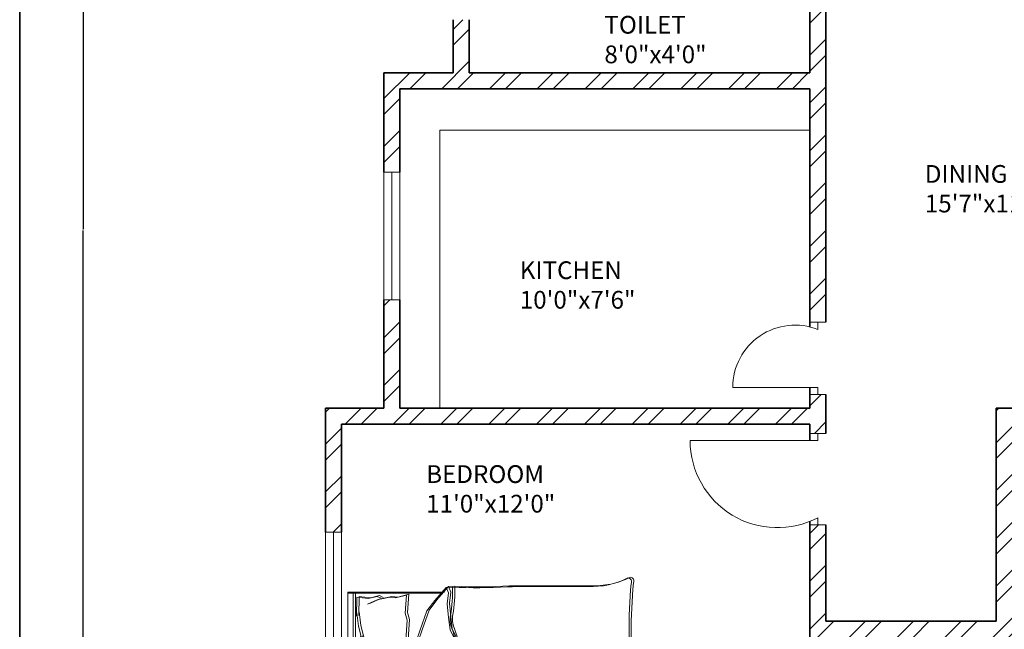
# Model space of a CAD drawing. Units: inches. Extents: x 1885 to 2748, y 783 to 2421.
# Tile 20 of 117: x 1885 to 2163, y 1178 to 1350. Entities that reach past the tile are written whole.
import ezdxf

# ---------------------------------------------------------------- set-up
doc = ezdxf.new("R2010")
doc.units = ezdxf.units.IN
for name, color, linetype, lineweight in [('A-ANNO-DIMS', 2, 'Continuous', 18), ('A-ANNO-TTLB', 7, 'Continuous', 35), ('A-AREA-IDEN', 7, 'Continuous', 18), ('A-DOOR', 31, 'Continuous', 18), ('A-FLOR-CASE', 9, 'Continuous', 18), ('A-FURN', 8, 'Continuous', 13), ('A-GLAZ', 181, 'Continuous', 18), ('A-WALL', 7, 'Continuous', 35)]:
    doc.layers.add(name, color=color, linetype=linetype, lineweight=lineweight)
doc.layers.add('A-WALL-PATT', color=85, linetype='Continuous', lineweight=13, true_color=0x58ba48)
doc.styles.get("Standard").update_dxf_attribs({"font": 'arial.ttf'})
doc.dimstyles.get("Standard").update_dxf_attribs({"dimtxt": 0.18, "dimasz": 0.18, "dimexe": 0.18, "dimexo": 0.0625, "dimgap": 0.09, "dimtad": 0, "dimtih": 1, "dimtoh": 1, "dimdec": 4, "dimzin": 0, "dimdsep": 46, "dimtxsty": 'Standard', "dimcen": 0.09, "dimadec": 0, "dimazin": 0, "dimtfac": 1, "dimtdec": 4, "dimtofl": 0, "dimtmove": 0, "dimatfit": 3, "dimfxl": 1, "dimtolj": 1, "dimtzin": 0, "dimarcsym": 0})

# ---------------------------------------------------------------- blocks, each defined once
blk = doc.blocks.new('BED-DOUBLE')
for p, q in [((27.75, 52.87), (24.5, 49.16)), ((27.75, 52.87), (24.5, 49.16)), ((28.39, 53.09), (25.14, 49.39)), ((28.39, 53.09), (25.14, 49.39)), ((29.49, 52.95), (27.75, 52.87, 3.87)), ((29.49, 52.95), (27.75, 52.87, 3.87)), ((28.37, 51.33), (27.75, 52.87)), ((28.37, 51.33), (27.75, 52.87)), ((30.13, 53.17), (28.39, 53.09, 3.87)), ((30.13, 53.17), (28.39, 53.09, 3.87)), ((29.01, 51.56), (28.39, 53.09)), ((29.01, 51.56), (28.39, 53.09)), ((0, 51.49), (0.64, 51.49)), ((0, 3.47), (0, 51.49)), ((0, 51.26), (26.61, 51.26)), ((0, 51.26), (26.61, 51.26)), ((0.64, 51.49), (27.25, 51.49)), ((0.64, 51.49), (27.25, 51.49)), ((1.54, 3.47), (1.54, 51.26)), ((1.54, 3.47), (1.54, 51.26)), ((2.18, 3.7), (2.18, 51.49)), ((2.18, 3.7), (2.18, 51.49)), ((2.56, 50.11), (2.46, 44.71)), ((2.56, 50.11), (2.46, 44.71)), ((2.56, 50.11), (5.77, 49.73)), ((2.56, 50.11), (5.77, 49.73)), ((3.2, 50.34), (3.1, 44.94)), ((3.2, 50.34), (3.1, 44.94)), ((3.2, 50.34), (6.41, 49.96)), ((3.2, 50.34), (6.41, 49.96)), ((5.77, 49.73), (8.34, 50.33)), ((5.77, 49.73), (8.34, 50.33)), ((6.41, 49.96), (8.98, 50.56)), ((6.41, 49.96), (8.98, 50.56)), ((11.83, 50.11), (8.26, 49.31)), ((11.83, 50.11), (8.26, 49.31)), ((8.34, 50.33), (9.39, 49.81)), ((8.34, 50.33), (9.39, 49.81)), ((12.47, 50.34), (8.9, 49.54)), ((12.47, 50.34), (8.9, 49.54)), ((8.98, 50.56), (10.03, 50.04)), ((8.98, 50.56), (10.03, 50.04)), ((13.44, 49.92), (11.83, 50.11)), ((13.44, 49.92), (11.83, 50.11)), ((14.08, 50.15), (12.47, 50.34)), ((14.08, 50.15), (12.47, 50.34)), ((16.58, 50.7), (13.44, 49.92)), ((16.58, 50.7), (13.44, 49.92)), ((17.22, 50.93), (14.08, 50.15)), ((17.22, 50.93), (14.08, 50.15)), ((16.17, 45.57), (16.58, 50.7)), ((16.17, 45.56), (16.58, 50.7)), ((16.81, 45.79), (17.22, 50.93)), ((16.81, 45.79), (17.22, 50.93)), ((28.06, 48.23), (28.37, 51.33)), ((28.06, 48.23), (28.37, 51.33)), ((28.7, 48.46), (29.01, 51.56)), ((28.7, 48.46), (29.01, 51.56)), ((8.26, 49.31), (5.58, 48.13)), ((8.26, 49.31), (5.58, 48.13)), ((8.9, 49.54), (6.22, 48.36)), ((8.9, 49.54), (6.22, 48.36)), ((24.5, 49.16), (22.33, 46.22)), ((24.5, 49.16), (22.33, 46.22)), ((25.14, 49.39), (22.97, 46.45)), ((25.14, 49.39), (22.97, 46.45)), ((28.37, 44.36), (28.06, 48.23)), ((28.37, 44.36), (28.06, 48.23)), ((29.01, 44.59), (28.7, 48.46)), ((29.01, 44.59), (28.7, 48.46)), ((2.46, 44.71), (2.55, 45.71)), ((2.46, 44.71), (2.55, 45.71)), ((2.55, 45.71), (3.07, 41.91)), ((2.55, 45.71), (3.07, 41.91)), ((3.1, 44.94), (3.19, 45.94)), ((3.1, 44.94), (3.19, 45.94)), ((3.19, 45.94), (3.71, 42.14)), ((3.19, 45.94), (3.71, 42.14)), ((16.73, 43.6), (16.17, 45.57)), ((16.73, 43.6), (16.17, 45.56)), ((17.37, 43.83), (16.81, 45.79)), ((17.37, 43.83), (16.81, 45.79)), ((22.33, 46.22), (20.32, 40.64)), ((22.33, 46.22), (20.32, 40.64)), ((22.97, 46.45), (20.96, 40.87)), ((22.97, 46.45), (20.96, 40.87)), ((29.47, 41.18), (29.01, 44.59)), ((29.47, 41.18), (29.01, 44.59)), ((3.07, 41.91), (4.43, 36.49)), ((3.07, 41.91), (4.43, 36.49)), ((3.71, 42.14), (5.07, 36.72)), ((3.71, 42.14), (5.07, 36.72)), ((16.3, 36.59), (16.73, 43.6)), ((16.3, 36.59), (16.73, 43.6)), ((16.94, 36.82), (17.37, 43.83)), ((16.94, 36.82), (17.37, 43.83)), ((28.83, 40.95), (28.37, 44.36)), ((28.83, 40.95), (28.37, 44.36)), ((3.68, 39.2), (3.08, 37.13)), ((3.68, 39.2), (3.08, 37.13)), ((4.32, 39.43), (3.72, 37.36)), ((4.32, 39.43), (3.72, 37.36)), ((20.32, 40.64), (17.39, 32.3)), ((20.32, 40.64), (17.39, 32.3)), ((20.96, 40.87), (18.03, 32.53)), ((20.96, 40.87), (18.03, 32.53)), ((29.76, 38.94), (28.83, 40.95)), ((29.76, 38.94), (28.83, 40.95)), ((30.4, 39.17), (29.47, 41.18)), ((30.4, 39.17), (29.47, 41.18)), ((30.38, 36.46), (29.76, 38.94)), ((30.38, 36.46), (29.76, 38.94)), ((31.02, 36.69), (30.4, 39.17)), ((31.02, 36.69), (30.4, 39.17)), ((79.25, 15.06), (79.25, 39.68)), ((79.25, 15.06), (79.25, 39.68)), ((79.89, 15.29), (79.89, 39.9)), ((79.89, 15.29), (79.89, 39.9)), ((3.08, 37.13), (2.54, 34.2)), ((3.08, 37.13), (2.54, 34.2)), ((3.72, 37.36), (3.18, 34.43)), ((3.72, 37.36), (3.18, 34.43)), ((15.63, 32.56), (16.3, 36.59)), ((15.63, 32.56), (16.3, 36.59)), ((16.27, 32.79), (16.94, 36.82)), ((16.27, 32.79), (16.94, 36.82)), ((23.88, 34.45), (28.37, 36.15)), ((23.88, 34.45), (28.37, 36.15)), ((24.52, 34.68), (29.01, 36.38)), ((24.52, 34.68), (29.01, 36.38)), ((28.37, 36.15), (30.38, 36.46)), ((28.37, 36.15), (30.38, 36.46)), ((29.01, 36.38), (31.02, 36.69)), ((29.01, 36.38), (31.02, 36.69)), ((2.54, 34.2), (2.56, 33.88)), ((2.54, 34.2), (2.56, 33.88)), ((2.56, 33.88), (2.98, 29.45)), ((2.56, 33.88), (2.98, 29.45)), ((3.18, 34.43), (3.2, 34.11)), ((3.18, 34.43), (3.2, 34.11)), ((3.2, 34.11), (3.62, 29.68)), ((3.2, 34.11), (3.62, 29.68)), ((16.74, 30.75), (15.46, 33.82)), ((16.74, 30.75), (15.46, 33.82)), ((17.38, 30.98), (16.1, 34.05)), ((17.38, 30.98), (16.1, 34.05)), ((17.39, 30.26), (23.88, 34.45)), ((17.39, 30.26), (23.88, 34.45)), ((18.03, 30.49), (24.52, 34.68)), ((18.03, 30.49), (24.52, 34.68)), ((16.9, 28.3), (16.74, 30.75)), ((16.9, 28.3), (16.74, 30.75)), ((17.54, 28.52), (17.38, 30.98)), ((17.54, 28.52), (17.38, 30.98)), ((2.98, 29.45), (2.5, 27.98)), ((2.98, 29.45), (2.5, 27.98)), ((2.5, 27.98), (7.87, 27.73)), ((2.5, 27.98), (7.87, 27.73)), ((3.62, 29.68), (3.13, 28.2)), ((3.62, 29.68), (3.13, 28.2)), ((3.13, 28.2), (8.51, 27.96)), ((3.13, 28.2), (8.51, 27.96)), ((8.51, 27.96), (11.72, 27.58)), ((8.51, 27.96), (11.72, 27.58)), ((12.38, 27.43), (14.22, 28.13)), ((12.38, 27.43), (14.22, 28.13)), ((13.02, 27.66), (14.86, 28.36)), ((13.02, 27.66), (14.86, 28.36)), ((14.22, 28.13), (16.9, 28.3)), ((14.22, 28.13), (16.9, 28.3)), ((14.86, 28.36), (17.54, 28.52)), ((14.86, 28.36), (17.54, 28.52)), ((1.87, 25.98), (7.22, 26.56)), ((1.87, 25.98), (7.22, 26.56)), ((2.45, 24.54), (1.87, 25.98)), ((2.45, 24.54), (1.87, 25.98)), ((2.51, 26.21), (7.86, 26.79)), ((2.51, 26.21), (7.86, 26.79)), ((3.09, 24.76), (2.51, 26.21)), ((3.09, 24.76), (2.51, 26.21)), ((7.22, 26.56), (10.4, 27.14)), ((7.22, 26.56), (10.4, 27.14)), ((7.86, 26.79), (11.04, 27.37)), ((7.86, 26.79), (11.04, 27.37)), ((7.87, 27.73), (11.08, 27.35)), ((7.87, 27.73), (11.08, 27.35)), ((10.4, 27.14), (11.71, 27.14)), ((10.4, 27.14), (11.71, 27.14)), ((11.04, 27.37), (12.35, 27.37)), ((11.04, 27.37), (12.35, 27.37)), ((11.08, 27.35), (12.38, 27.43)), ((11.08, 27.35), (12.38, 27.43)), ((11.71, 27.14), (13.59, 26.56)), ((11.71, 27.14), (13.59, 26.56)), ((11.72, 27.58), (13.02, 27.66)), ((11.72, 27.58), (13.02, 27.66)), ((12.35, 27.37), (14.22, 26.79)), ((12.35, 27.37), (14.22, 26.79)), ((13.59, 26.56), (16.27, 26.56)), ((13.59, 26.56), (16.27, 26.56)), ((14.22, 26.79), (16.91, 26.79)), ((14.22, 26.79), (16.91, 26.79)), ((16.27, 26.56), (16.27, 24.1)), ((16.27, 26.56), (16.27, 24.1)), ((16.91, 26.79), (16.91, 24.33)), ((16.91, 26.79), (16.91, 24.33)), ((2.31, 20.09), (2.45, 24.54)), ((2.31, 20.09), (2.45, 24.54)), ((2.95, 20.32), (3.09, 24.76)), ((2.95, 20.32), (3.09, 24.76)), ((16.27, 24.1), (15.18, 20.96)), ((16.27, 24.1), (15.18, 20.96)), ((16.91, 24.33), (15.82, 21.19)), ((16.91, 24.33), (15.82, 21.19)), ((16.17, 19.38), (16.58, 24.51)), ((16.17, 19.38), (16.58, 24.51)), ((16.81, 19.61), (17.22, 24.74)), ((16.81, 19.61), (17.22, 24.74)), ((2.31, 19.77), (2.31, 20.09)), ((2.31, 19.77), (2.31, 20.09)), ((3.03, 16.88), (2.31, 19.77)), ((3.03, 16.88), (2.31, 19.77)), ((2.95, 20), (2.95, 20.32)), ((2.95, 20), (2.95, 20.32)), ((3.67, 17.11), (2.95, 20)), ((3.67, 17.11), (2.95, 20)), ((17.37, 17.65), (16.81, 19.61)), ((17.37, 17.65), (16.81, 19.61)), ((3.75, 14.85), (3.03, 16.88)), ((3.75, 14.85), (3.03, 16.88)), ((3.32, 12.11), (4.33, 17.6)), ((3.32, 12.11), (4.33, 17.6)), ((4.39, 15.08), (3.67, 17.11)), ((4.39, 15.08), (3.67, 17.11)), ((3.96, 12.34), (4.97, 17.83)), ((3.96, 12.34), (4.97, 17.83)), ((16.73, 17.42), (16.17, 19.38)), ((16.73, 17.42), (16.17, 19.38)), ((16.3, 10.41), (16.73, 17.42)), ((16.3, 10.41), (16.73, 17.42)), ((16.94, 10.64), (17.37, 17.65)), ((16.94, 10.64), (17.37, 17.65)), ((3.03, 8.28), (3.32, 12.11)), ((3.03, 8.28), (3.32, 12.11)), ((3.67, 8.51), (3.96, 12.34)), ((3.67, 8.51), (3.96, 12.34)), ((3.65, 8.41), (3.67, 8.51)), ((3.65, 8.41), (3.67, 8.51)), ((3.98, 4.13), (3.65, 8.41)), ((3.98, 4.13), (3.65, 8.41)), ((15.63, 6.38), (16.3, 10.41)), ((15.63, 6.38), (16.3, 10.41)), ((16.27, 6.61), (16.94, 10.64)), ((16.27, 6.61), (16.94, 10.64)), ((16.3, 10.41), (16.62, 9.28)), ((16.3, 10.41), (16.62, 9.28)), ((16.62, 9.28), (17.34, 4.18)), ((16.62, 9.28), (17.34, 4.18)), ((16.94, 10.64), (17.26, 9.51)), ((16.94, 10.64), (17.26, 9.51)), ((17.26, 9.51), (17.98, 4.41)), ((17.26, 9.51), (17.98, 4.41)), ((3.01, 8.18), (3.03, 8.28)), ((3.01, 8.18), (3.03, 8.28)), ((3.34, 3.9), (3.01, 8.18)), ((3.34, 3.9), (3.01, 8.18)), ((8.96, 5.05), (6.21, 6.06)), ((8.96, 5.05), (6.21, 6.06)), ((9.6, 5.28), (6.85, 6.29)), ((9.6, 5.28), (6.85, 6.29)), ((18.11, 3.47), (0, 3.47)), ((18.11, 3.47), (0, 3.47)), ((18.75, 3.7), (0.64, 3.7)), ((18.75, 3.7), (0.64, 3.7)), ((3.32, 3.89), (6.5, 4.47)), ((3.32, 3.89), (6.5, 4.47)), ((3.96, 4.12), (7.14, 4.7)), ((3.96, 4.12), (7.14, 4.7)), ((6.5, 4.47), (9.1, 4.04)), ((6.5, 4.47), (9.1, 4.04)), ((7.14, 4.7), (9.74, 4.27)), ((7.14, 4.7), (9.74, 4.27)), ((12.57, 4.47), (8.96, 5.05)), ((12.57, 4.47), (8.96, 5.05)), ((9.1, 4.04), (10.12, 4.62)), ((9.1, 4.04), (10.12, 4.62)), ((13.21, 4.7), (9.6, 5.28)), ((13.21, 4.7), (9.6, 5.28)), ((9.74, 4.27), (10.75, 4.84)), ((9.74, 4.27), (10.75, 4.84)), ((14.16, 4.76), (12.57, 4.47)), ((14.16, 4.76), (12.57, 4.47)), ((14.8, 4.99), (13.21, 4.7)), ((14.8, 4.99), (13.21, 4.7)), ((17.34, 4.18), (14.16, 4.76)), ((17.34, 4.18), (14.16, 4.76)), ((17.98, 4.41), (14.8, 4.99)), ((17.98, 4.41), (14.8, 4.99))]:
    blk.add_line(p, q)
for centre, radius, start, end in [((68.67, 76.16), 23.07, 267.4714, 296.4681), ((68.67, 76.16), 23.07, 267.4714, 296.4681), ((69.31, 76.38), 23.07, 267.4714, 296.4681), ((69.31, 76.38), 23.07, 267.4714, 296.4681), ((78.87, 54.41), 1.1, 332.6588, 86.02), ((78.87, 54.41), 1.1, 332.6588, 86.02), ((79.51, 54.64), 1.1, 332.6588, 86.02), ((79.51, 54.64), 1.1, 332.6588, 86.02), ((-6.65, 51.33), 36.18, 349.8763, 2.5657), ((-6.65, 51.33), 36.18, 349.8763, 2.5657), ((36.32, 182.26), 129.5, 266.9791, 273.8365), ((36.32, 182.26), 129.5, 266.9791, 273.8365), ((-6.01, 51.55), 36.18, 349.8763, 2.5657), ((-6.01, 51.55), 36.18, 349.8763, 2.5657), ((36.96, 182.49), 129.5, 266.9791, 273.8365), ((36.96, 182.49), 129.5, 266.9791, 273.8365), ((67.83, -4508.74), 4561.86, 90.00217, 90.28689), ((67.83, -4508.75), 4561.86, 90.00217, 90.28689), ((68.46, -4508.52), 4561.86, 90.00217, 90.28689), ((68.46, -4508.52), 4561.86, 90.00217, 90.28689), ((212.28, 41.15), 133.04, 174.4998, 180.6351), ((212.28, 41.15), 133.04, 174.4998, 180.6351), ((212.92, 41.38), 133.04, 174.4998, 180.6351), ((212.92, 41.38), 133.04, 174.4998, 180.6351), ((35.07, 43.74), 6.22, 168.6608, 203.7384), ((35.07, 43.74), 6.22, 168.6608, 203.7384), ((35.71, 43.97), 6.22, 168.6608, 203.7384), ((35.71, 43.97), 6.22, 168.6608, 203.7384), ((1.49, 31.15), 29.65, 10.6617, 19.8806), ((1.49, 31.15), 29.65, 10.6617, 19.8806), ((2.13, 31.38), 29.65, 10.6617, 19.8806), ((2.13, 31.38), 29.65, 10.6617, 19.8806), ((156.32, 17.75), 129.02, 171.7845, 186.9006), ((156.32, 17.75), 129.02, 171.7845, 186.9006), ((156.96, 17.98), 129.02, 171.7845, 186.9006), ((156.96, 17.98), 129.02, 171.7845, 186.9006), ((30.44, 36.64), 0.185, 250.2464, 1.1377), ((30.44, 36.63), 0.185, 250.2464, 1.1377), ((31.08, 36.86), 0.185, 250.2464, 1.1377), ((31.08, 36.86), 0.185, 250.2464, 1.1377), ((182.06, 21.36), 164.97, 176.0865, 186.7821), ((182.06, 21.36), 164.97, 176.0865, 186.7821), ((182.7, 21.59), 164.97, 176.0865, 186.7821), ((182.7, 21.59), 164.97, 176.0865, 186.7821), ((-23.71, -17.22), 106.46, 13.3832, 17.7053), ((-23.71, -17.22), 106.46, 13.3832, 17.7053), ((-23.07, -16.99), 106.46, 13.3832, 17.7053), ((-23.07, -16.99), 106.46, 13.3832, 17.7053), ((200.84, 21.43), 121.76, 182.9958, 189.4091), ((200.84, 21.43), 121.76, 182.9958, 189.4091), ((201.48, 21.65), 121.76, 182.9958, 189.4091), ((201.48, 21.65), 121.76, 182.9958, 189.4091), ((31.18, -167.31), 170.11, 88.4762, 91.0082), ((31.18, -167.31), 170.11, 88.4762, 91.0082), ((31.82, -167.08), 170.11, 88.4762, 91.0082), ((31.82, -167.08), 170.11, 88.4762, 91.0082), ((51.26, 485.05), 482.31, 268.2277, 271.7185), ((51.26, 485.05), 482.31, 268.2277, 271.7185), ((65.16, -26.67), 29.63, 76.0648, 88.9113), ((65.16, -26.67), 29.63, 76.0648, 88.9113), ((20.1, 85.16), 83.31, 268.7218, 275.604), ((20.1, 85.16), 83.31, 268.7218, 275.604), ((20.74, 85.39), 83.31, 268.7218, 275.604), ((20.74, 85.39), 83.31, 268.7218, 275.604), ((50.62, 484.82), 482.31, 268.2277, 271.7185), ((50.62, 484.82), 482.31, 268.2277, 271.7185), ((64.52, -26.9), 29.63, 76.0648, 88.9113), ((64.52, -26.9), 29.63, 76.0648, 88.9113), ((70.28, -21.66), 23.56, 67.9751, 86.652), ((70.28, -21.66), 23.56, 67.9751, 86.652), ((70.92, -21.43), 23.56, 67.9751, 86.652), ((70.92, -21.43), 23.56, 67.9751, 86.652), ((79.72, 1.09), 1.09, 236.1736, 23.4781), ((79.72, 1.09), 1.09, 236.1736, 23.4781), ((80.36, 1.31), 1.09, 236.1736, 23.4781), ((80.36, 1.31), 1.09, 236.1736, 23.4781)]:
    blk.add_arc(centre, radius, start, end)
blk = doc.blocks.new('WIN-60')
for p, q in [((0, 60), (4.5, 60)), ((0, 60), (0, 0)), ((4.5, 60), (2.25, 60)), ((2.25, 60), (2.25, 0)), ((4.5, 0), (4.5, 60)), ((2.25, 0), (0, 0)), ((0, 0), (4.5, 0))]:
    blk.add_line(p, q)
blk = doc.blocks.new('WIN-36-ALT')
for p, q in [((0, 36), (4.5, 36)), ((0, 36), (0, 0)), ((4.5, 36), (2.25, 36)), ((2.25, 36), (2.25, 0)), ((4.5, 0), (4.5, 36)), ((4.5, 0), (0, 0)), ((2.25, 0), (4.5, 0))]:
    blk.add_line(p, q)
blk = doc.blocks.new('*D45')
at = {"layer": 'A-ANNO-DIMS', "color": 0, "lineweight": -2, "transparency": 16777216}
for p, q in [((1980.71, 1524.01), (1902.84, 1524.01)), ((1903.02, 1523.83), (1903.02, 1290.94)), ((1903.02, 1057.69), (1903.02, 1290.57)), ((1971.21, 1057.51), (1902.84, 1057.51))]:
    blk.add_line(p, q, dxfattribs=at)
at = {"layer": 'A-ANNO-DIMS', "color": 0, "transparency": 16777216}
for points in [[(1902.99, 1523.83), (1903.05, 1523.83), (1903.02, 1524.01)], [(1902.99, 1057.69), (1903.05, 1057.69), (1903.02, 1057.51)]]:
    blk.add_solid(points, dxfattribs=at)
at = {"layer": 'Defpoints', "color": 0, "transparency": 16777216}
for p in [(1903.02, 1524.01), (1980.77, 1524.01), (1971.27, 1057.51)]:
    blk.add_point(p, dxfattribs=at)
at = {"layer": 'A-ANNO-DIMS', "color": 0, "transparency": 16777216, "insert": (1903.02, 1290.76), "char_height": 0.18, "attachment_point": 5}
blk.add_mtext('\\A1;466.5', dxfattribs=at)

msp = doc.modelspace()

# ---------------------------------------------------------------- hatches: boundary and pattern name
at = {"layer": 'A-WALL-PATT'}
h = msp.add_hatch(dxfattribs=at)
h.set_pattern_fill('ANSI32', color=256)
h.paths.add_polyline_path([(2007.77, 2318.01), (1980.77, 2318.01), (1980.77, 2281.22), (1985.27, 2281.22), (1985.27, 2313.51), (2007.77, 2313.51), (2007.77, 2315.76)])
h.paths.add_polyline_path([(2094.32, 2318.01), (2067.77, 2318.01), (2067.77, 2313.51), (2094.32, 2313.51), (2094.32, 2315.76)])
h.paths.add_polyline_path([(2131.37, 2315.76), (2131.37, 2318.01), (2131.19, 2318.01), (2112.61, 2318.01), (2112.61, 2313.51), (2117.27, 2313.51), (2117.27, 2255.2), (2121.77, 2255.2), (2121.77, 2313.51), (2131.37, 2313.51)])
h.paths.add_polyline_path([(2190.51, 2318.01), (2155.37, 2318.01), (2155.37, 2313.51), (2169.77, 2313.51), (2169.77, 2229.51), (2121.77, 2229.51), (2121.77, 2233.45), (2119.52, 2233.45), (2117.27, 2233.45), (2117.27, 2201.1), (2121.77, 2201.1), (2121.77, 2225.01), (2169.77, 2225.01), (2169.77, 2165.01), (2306.27, 2165.01), (2306.27, 2066.01), (2310.77, 2066.01), (2344.27, 2066.01), (2486.27, 2066.01), (2486.27, 1886.01), (2483.02, 1886.01), (2483.02, 1881.51), (2486.27, 1881.51), (2486.27, 1880.68), (2490.77, 1880.68), (2490.77, 2070.51), (2344.27, 2070.51), (2310.77, 2070.51), (2310.77, 2165.01), (2310.77, 2173.64), (2308.52, 2173.64), (2306.27, 2173.64), (2306.27, 2169.51), (2174.27, 2169.51), (2174.27, 2313.51), (2190.51, 2313.51), (2190.51, 2315.76)])
h.paths.add_polyline_path([(1985.27, 2221.22), (1980.77, 2221.22), (1980.77, 2165.01), (1992.77, 2165.01), (1992.77, 2141.93), (1997.27, 2141.93), (1997.27, 2165.01), (2117.27, 2165.01), (2117.27, 2163.13), (2121.77, 2163.13), (2121.77, 2172.73), (2119.52, 2172.73), (2117.27, 2172.73), (2117.27, 2169.51), (1985.27, 2169.51)])
h.paths.add_polyline_path([(1997.27, 2105.93), (1992.77, 2105.93), (1992.77, 2070.51), (2016.77, 2070.51), (2016.77, 2059.12), (2019.02, 2059.12), (2021.27, 2059.12), (2021.27, 2070.51), (2117.27, 2070.51), (2117.27, 2022.51), (2114.42, 2022.51), (2114.42, 2018.01), (2123.63, 2018.01), (2123.63, 2020.26), (2123.63, 2022.51), (2121.77, 2022.51), (2121.77, 2142.59), (2119.52, 2142.59), (2117.27, 2142.59), (2117.27, 2075.01), (1997.27, 2075.01)])
h.paths.add_polyline_path([(2092.03, 2020.26), (2092.03, 2022.51), (2021.27, 2022.51), (2021.27, 2035.12), (2016.77, 2035.12), (2016.77, 2018.01), (2016.77, 1978.78), (2021.27, 1978.78), (2021.27, 2018.01), (2092.03, 2018.01)])
h.paths.add_polyline_path([(2260.94, 2022.51), (2153.1, 2022.51), (2153.1, 2020.26), (2153.1, 2018.01), (2155.27, 2018.01), (2155.27, 1886.01), (2107.63, 1886.01), (2107.63, 1881.51), (2182.91, 1881.51), (2182.91, 1883.76), (2182.91, 1886.01), (2159.77, 1886.01), (2159.77, 2018.01), (2260.94, 2018.01), (2260.94, 2020.26)])
h.paths.add_polyline_path([(2047.63, 1883.76), (2047.63, 1886.01), (2021.27, 1886.01), (2021.27, 1918.78), (2019.02, 1918.78), (2016.77, 1918.78), (2016.77, 1881.51), (2047.63, 1881.51)])
h.paths.add_polyline_path([(2306.36, 1883.76), (2306.36, 1886.01), (2296.27, 1886.01), (2296.27, 1982.01), (2316.54, 1982.01), (2316.54, 1984.26), (2316.54, 1986.51), (2296.27, 1986.51), (2296.27, 2022.51), (2289.28, 2022.51), (2289.28, 2018.01), (2291.77, 2018.01), (2291.77, 1886.01), (2242.91, 1886.01), (2242.91, 1881.51), (2306.36, 1881.51)], flags=17)
h.paths.add_polyline_path([(1985.27, 1843.01), (2021.6, 1843.01), (2021.53, 1845.44), (2021.48, 1847.51), (1980.77, 1847.51), (1980.77, 1809.45), (1985.27, 1809.45)])
h.paths.add_polyline_path([(2131.48, 1845.26), (2131.48, 1847.51), (2081.53, 1847.51), (2081.53, 1843.01), (2117.27, 1843.01), (2117.27, 1784.15), (2119.52, 1784.15), (2121.77, 1784.15), (2121.77, 1843.01), (2131.48, 1843.01)])
h.paths.add_polyline_path([(2203.89, 1847.51), (2155.48, 1847.51), (2155.48, 1843.01), (2169.77, 1843.01), (2169.77, 1759.01), (2121.77, 1759.01), (2121.77, 1761.46), (2117.27, 1761.46), (2117.27, 1730.43), (2121.77, 1730.43), (2121.77, 1754.51), (2177.42, 1754.51), (2177.42, 1756.76), (2177.42, 1759.01), (2174.27, 1759.01), (2174.27, 1843.01), (2203.89, 1843.01)])
h.paths.add_polyline_path([(2335.55, 1845.26), (2335.55, 1847.51), (2239.89, 1847.51), (2239.89, 1843.01), (2306.27, 1843.01), (2306.27, 1759.01), (2199.49, 1759.01), (2199.49, 1754.51), (2310.77, 1754.51), (2310.77, 1843.01), (2335.55, 1843.01)])
h.paths.add_polyline_path([(2348.77, 2022.51), (2344.27, 2022.51), (2344.27, 1986.51), (2341.68, 1986.51), (2341.68, 1982.01), (2344.27, 1982.01), (2344.27, 1886.01), (2330.36, 1886.01), (2330.36, 1881.51), (2361.63, 1881.51), (2361.63, 1883.76), (2361.63, 1886.01), (2348.77, 1886.01)], flags=17)
h.paths.add_polyline_path([(2283.25, 2315.76), (2283.25, 2318.01), (2238.51, 2318.01), (2238.51, 2313.51), (2283.25, 2313.51)], flags=17)
h.paths.add_polyline_path([(2363.27, 2348.01), (2388.68, 2348.01), (2388.68, 2350.26), (2388.68, 2352.51), (2358.77, 2352.51), (2358.77, 2348.01), (2358.77, 2318.01), (2344.48, 2318.01), (2344.48, 2313.51), (2358.77, 2313.51), (2358.77, 2229.51), (2310.77, 2229.51), (2310.77, 2231.95), (2306.27, 2231.95), (2306.27, 2205.61), (2310.77, 2205.61), (2310.77, 2225.01), (2358.77, 2225.01), (2358.77, 2211.51), (2452.33, 2211.51), (2452.33, 2213.76), (2452.33, 2216.01), (2363.27, 2216.01), (2363.27, 2318.01)])
h.paths.add_polyline_path([(2310.77, 2313.51), (2320.48, 2313.51), (2320.48, 2315.76), (2320.48, 2318.01), (2302.73, 2318.01), (2302.73, 2313.51), (2306.27, 2313.51), (2306.27, 2251.08), (2310.77, 2251.08)], flags=17)
h.paths.add_polyline_path([(2490.77, 2352.51), (2486.27, 2352.51), (2448.68, 2352.51), (2448.68, 2348.01), (2486.27, 2348.01), (2486.27, 2318.01), (2486.27, 2216.01), (2481.78, 2216.01), (2481.78, 2211.51), (2486.27, 2211.51), (2486.27, 2165.01), (2493.29, 2165.01), (2493.29, 2167.26), (2493.29, 2169.51), (2490.77, 2169.51), (2490.77, 2313.51), (2494.43, 2313.51), (2494.43, 2318.01), (2490.77, 2318.01)])
h.paths.add_polyline_path([(2534.65, 2318.01), (2515.69, 2318.01), (2515.69, 2313.51), (2534.65, 2313.51), (2534.65, 2315.76)])
h.paths.add_polyline_path([(2618.27, 2318.01), (2594.65, 2318.01), (2594.65, 2313.51), (2613.77, 2313.51), (2613.77, 2281.71), (2618.27, 2281.71)])
h.paths.add_polyline_path([(2618.27, 2221.71), (2613.77, 2221.71), (2613.77, 2169.51), (2554.02, 2169.51), (2554.02, 2165.01), (2613.77, 2165.01), (2613.77, 2152.88), (2618.27, 2152.88)])
h.paths.add_polyline_path([(2618.27, 2128.88), (2616.02, 2128.88), (2613.77, 2128.88), (2613.77, 2117.01), (2529.77, 2117.01), (2529.77, 2165.01), (2532.85, 2165.01), (2532.85, 2169.51), (2522.87, 2169.51), (2522.87, 2165.01), (2525.27, 2165.01), (2525.27, 2117.01), (2525.27, 2112.51), (2525.27, 2108.58), (2529.77, 2108.58), (2529.77, 2112.51), (2613.77, 2112.51), (2613.77, 2080.19), (2618.27, 2080.19)])
h.paths.add_polyline_path([(2618.27, 2044.19), (2616.02, 2044.19), (2613.77, 2044.19), (2613.77, 2015.51), (2529.77, 2015.51), (2529.77, 2088.58), (2527.52, 2088.58), (2525.27, 2088.58), (2525.27, 2011.01), (2613.77, 2011.01), (2613.77, 1956.75), (2618.27, 1956.75)])
h.paths.add_polyline_path([(2618.27, 1881.51), (2618.27, 1896.75), (2613.77, 1896.75), (2613.77, 1881.51), (2613.77, 1847.51), (2592.71, 1847.51), (2592.71, 1843.01), (2613.77, 1843.01), (2613.77, 1765.01), (2613.77, 1760.51), (2609.62, 1760.51), (2609.62, 1756.01), (2613.77, 1756.01), (2613.77, 1660.01), (2608.54, 1660.01), (2608.54, 1655.51), (2613.77, 1655.51), (2613.77, 1508.16), (2618.27, 1508.16)])
h.paths.add_polyline_path([(2565.77, 1843.01), (2569, 1843.01), (2569, 1847.51), (2490.77, 1847.51), (2490.77, 1849.7), (2488.52, 1849.7), (2486.27, 1849.7), (2486.27, 1847.51), (2477.27, 1847.51), (2477.27, 1838.51), (2477.27, 1821.49), (2486.27, 1821.49), (2486.27, 1838.51), (2561.27, 1838.51), (2561.27, 1765.01), (2486.27, 1765.01), (2486.27, 1786.16), (2477.27, 1786.16), (2477.27, 1765.01), (2477.27, 1756.01), (2486.27, 1756.01), (2565.77, 1756.01), (2585.62, 1756.01), (2585.62, 1758.26), (2585.62, 1760.51), (2565.77, 1760.51), (2565.77, 1765.01)])
h.paths.add_polyline_path([(2486.27, 1651.01), (2561.27, 1651.01), (2561.27, 1567.01), (2486.27, 1567.01), (2486.27, 1591.32), (2477.27, 1591.32), (2477.27, 1567.01), (2477.27, 1558.01), (2477.27, 1555.44), (2481.77, 1555.44), (2481.77, 1558.01), (2568.65, 1558.01), (2568.65, 1560.26), (2568.65, 1562.51), (2565.77, 1562.51), (2565.77, 1655.51), (2584.54, 1655.51), (2584.54, 1657.76), (2584.54, 1660.01), (2565.77, 1660.01), (2486.27, 1660.01), (2477.27, 1660.01), (2477.27, 1651.01), (2477.27, 1632.99), (2486.27, 1632.99)])
h.paths.add_polyline_path([(2449.97, 1883.76), (2449.97, 1886.01), (2421.63, 1886.01), (2421.63, 1881.51), (2449.97, 1881.51)], flags=17)
h.paths.add_polyline_path([(2447.27, 1847.51), (2395.55, 1847.51), (2395.55, 1843.01), (2442.77, 1843.01), (2442.77, 1809.27), (2447.27, 1809.27)])
h.paths.add_polyline_path([(1985.27, 1749.45), (1980.77, 1749.45), (1980.77, 1694.5), (1985.27, 1694.5), (1985.27, 1694.51), (1986.9, 1694.51), (1986.9, 1697.78), (1986.9, 1699.01), (1985.27, 1699.01)])
h.paths.add_polyline_path([(2152.77, 1699.01), (2121.77, 1699.01), (2121.77, 1703.67), (2119.52, 1703.67), (2117.27, 1703.67), (2117.27, 1699.01), (2009.22, 1699.01), (2009.22, 1694.51), (2148.27, 1694.51), (2148.27, 1692.63), (2152.77, 1692.63)])
h.paths.add_polyline_path([(2016.27, 1694.51), (2011.77, 1694.51), (2011.77, 1558.01), (2040.81, 1558.01), (2040.81, 1560.26), (2040.81, 1562.51), (2016.27, 1562.51)])
h.paths.add_polyline_path([(2152.77, 1663.02), (2150.52, 1663.02), (2148.27, 1663.02), (2148.27, 1562.51), (2100.81, 1562.51), (2100.81, 1558.01), (2165.12, 1558.01), (2165.12, 1560.26), (2165.12, 1562.51), (2152.77, 1562.51), (2152.77, 1610.51), (2224.77, 1610.51), (2224.77, 1607.99), (2229.27, 1607.99), (2229.27, 1615.01), (2152.77, 1615.01)])
h.paths.add_polyline_path([(2238.61, 1560.26), (2238.61, 1562.51), (2229.27, 1562.51), (2229.27, 1588.76), (2227.02, 1588.76), (2224.77, 1588.77), (2224.77, 1562.51), (2189.12, 1562.51), (2189.12, 1558.01), (2238.61, 1558.01)])
h.paths.add_polyline_path([(2336.02, 1560.26), (2336.02, 1562.51), (2310.77, 1562.51), (2310.77, 1656.35), (2308.52, 1656.35), (2306.27, 1656.35), (2306.27, 1562.51), (2286.61, 1562.51), (2286.61, 1558.01), (2336.02, 1558.01)])
h.paths.add_polyline_path([(2447.27, 1690.97), (2445.02, 1690.97), (2442.77, 1690.97), (2442.77, 1687.01), (2306.27, 1687.01), (2306.27, 1680.75), (2310.77, 1680.75), (2310.77, 1682.51), (2442.77, 1682.51), (2442.77, 1562.51), (2396.02, 1562.51), (2396.02, 1558.01), (2447.27, 1558.01)])
h.paths.add_polyline_path([(2447.27, 1749.27), (2445.02, 1749.27), (2442.77, 1749.27), (2442.77, 1717.23), (2447.27, 1717.23)])
h.paths.add_polyline_path([(2044.67, 1521.76), (2044.67, 1524.01), (2007.27, 1524.01), (2007.27, 1503.49), (2009.52, 1503.49), (2011.77, 1503.49), (2011.77, 1519.51), (2044.67, 1519.51)])
h.paths.add_polyline_path([(2177.97, 1521.76), (2177.97, 1524.01), (2104.67, 1524.01), (2104.67, 1519.51), (2145.77, 1519.51), (2145.77, 1387.51), (2143.37, 1387.51), (2143.37, 1383.01), (2251.59, 1383.01), (2251.59, 1385.26), (2251.59, 1387.51), (2150.27, 1387.51), (2150.27, 1519.51), (2177.97, 1519.51)])
h.paths.add_polyline_path([(2298.7, 1524.01), (2237.97, 1524.01), (2237.97, 1519.51), (2282.27, 1519.51), (2282.27, 1387.51), (2279.68, 1387.51), (2279.68, 1383.01), (2286.77, 1383.01), (2286.77, 1419.01), (2312.45, 1419.01), (2312.45, 1421.26), (2312.45, 1423.51), (2286.77, 1423.51), (2286.77, 1519.51), (2298.7, 1519.51), (2298.7, 1521.72)], flags=17)
h.paths.add_polyline_path([(2361.9, 1521.76), (2361.9, 1524.01), (2322.7, 1524.01), (2322.7, 1519.51), (2334.77, 1519.51), (2334.77, 1423.51), (2331.93, 1423.51), (2331.93, 1419.01), (2334.77, 1419.01), (2334.77, 1387.51), (2334.77, 1383.23), (2339.27, 1383.23), (2339.27, 1387.51), (2339.27, 1519.51), (2361.9, 1519.51)], flags=17)
h.paths.add_polyline_path([(2447.27, 1521.76), (2447.27, 1524.01), (2421.9, 1524.01), (2421.9, 1519.51), (2447.27, 1519.51)], flags=17)
h.paths.add_polyline_path([(2481.77, 1529.6), (2479.52, 1529.6), (2477.27, 1529.6), (2477.27, 1524.01), (2474.49, 1524.01), (2474.49, 1519.51), (2477.27, 1519.51), (2477.27, 1334.51), (2296.77, 1334.51), (2296.77, 1240.51), (2160.27, 1240.51), (2160.27, 1180.51), (2112.27, 1180.51), (2112.27, 1207.69), (2110.02, 1207.69), (2107.77, 1207.69), (2107.77, 1171.61), (2112.27, 1171.61), (2112.27, 1176.01), (2160.27, 1176.01), (2160.27, 1092.01), (2144.22, 1092.01), (2144.22, 1087.51), (2189.5, 1087.51), (2189.5, 1089.76), (2189.5, 1092.01), (2164.77, 1092.01), (2164.77, 1236.01), (2296.77, 1236.01), (2296.77, 1231.91), (2301.27, 1231.91), (2301.27, 1330.01), (2481.77, 1330.01), (2481.77, 1387.51)])
h.paths.add_polyline_path([(2618.27, 1448.16), (2613.77, 1448.16), (2613.77, 1382.51), (2529.77, 1382.51), (2525.27, 1382.51), (2525.27, 1307.06), (2529.77, 1307.06), (2529.77, 1378.01), (2613.77, 1378.01), (2613.77, 1354.99), (2618.27, 1354.99)])
h.paths.add_polyline_path([(2618.27, 1318.99), (2613.77, 1318.99), (2613.77, 1281.01), (2529.77, 1281.01), (2529.77, 1283.79), (2527.52, 1283.79), (2525.27, 1283.79), (2525.27, 1228.51), (2516.79, 1228.51), (2516.79, 1224.01), (2533.48, 1224.01), (2533.48, 1226.26), (2533.48, 1228.51), (2529.77, 1228.51), (2529.77, 1276.51), (2613.77, 1276.51), (2613.77, 1266.02), (2618.27, 1266.02)])
h.paths.add_polyline_path([(2618.27, 1134.96), (2613.77, 1134.96), (2613.77, 1092.01), (2594.54, 1092.01), (2594.54, 1087.51), (2618.27, 1087.51)])
h.paths.add_polyline_path([(2534.54, 1092.01), (2509.77, 1092.01), (2509.77, 1087.51), (2534.54, 1087.51), (2534.54, 1089.76)])
h.paths.add_polyline_path([(2481.27, 1224.01), (2484.12, 1224.01), (2484.12, 1226.26), (2484.12, 1228.51), (2476.77, 1228.51), (2476.77, 1198.51), (2471.61, 1198.51), (2471.61, 1194.01), (2476.77, 1194.01), (2476.77, 1062.01), (2436.89, 1062.01), (2436.89, 1057.51), (2476.77, 1057.51), (2481.27, 1057.51), (2481.27, 1062.01), (2481.27, 1087.51), (2485.35, 1087.51), (2485.35, 1089.76), (2485.35, 1092.01), (2481.27, 1092.01), (2481.27, 1117.51)])
h.paths.add_polyline_path([(2439.9, 1198.51), (2349.27, 1198.51), (2349.27, 1194.01), (2349.27, 1180.51), (2301.27, 1180.51), (2301.27, 1201.9), (2299.02, 1201.9), (2296.77, 1201.9), (2296.77, 1172.34), (2299.02, 1172.34), (2301.27, 1172.34), (2301.27, 1176.01), (2349.27, 1176.01), (2349.27, 1092.01), (2334.45, 1092.01), (2334.45, 1087.51), (2349.27, 1087.51), (2349.27, 1057.51), (2353.77, 1057.51), (2376.89, 1057.51), (2376.89, 1059.76), (2376.89, 1062.01), (2353.77, 1062.01), (2353.77, 1087.51), (2353.77, 1180.51), (2353.77, 1194.01), (2439.9, 1194.01), (2439.9, 1196.26)])
h.paths.add_polyline_path([(2270.6, 1089.76), (2270.6, 1092.01), (2249.5, 1092.01), (2249.5, 1087.51), (2270.6, 1087.51)], flags=17)
h.paths.add_polyline_path([(2310.45, 1092.01), (2301.27, 1092.01), (2301.27, 1153.29), (2296.77, 1153.29), (2296.77, 1092.01), (2293.79, 1092.01), (2293.79, 1087.51), (2310.45, 1087.51), (2310.45, 1089.76)], flags=17)
h.paths.add_polyline_path([(2112.27, 1150.33), (2110.02, 1150.33), (2107.77, 1150.33), (2107.77, 1092.01), (2104.47, 1092.01), (2104.47, 1087.51), (2120.22, 1087.51), (2120.22, 1089.76), (2120.22, 1092.01), (2112.27, 1092.01)])
h.paths.add_polyline_path([(2082.17, 1092.01), (2058.14, 1092.01), (2058.14, 1087.51), (2082.17, 1087.51), (2082.17, 1089.76)])
h.paths.add_polyline_path([(1975.77, 1145.64), (1971.27, 1145.64), (1971.27, 1087.51), (1980.77, 1087.51), (1998.14, 1087.51), (1998.14, 1089.76), (1998.14, 1092.01), (1985.27, 1092.01), (1975.77, 1092.01)])
h.paths.add_polyline_path([(2112.27, 1244.38), (2110.02, 1244.38), (2107.77, 1244.38), (2107.77, 1240.51), (1992.27, 1240.51), (1992.27, 1271.01), (1987.77, 1271.01), (1987.77, 1240.51), (1980.77, 1240.51), (1975.77, 1240.51), (1971.27, 1240.51), (1971.27, 1205.64), (1975.77, 1205.64), (1975.77, 1236.01), (2107.77, 1236.01), (2107.77, 1233.44), (2112.27, 1233.44), (2112.27, 1236.01)])
h.paths.add_polyline_path([(2112.27, 1383.01), (2114.78, 1383.01), (2114.78, 1385.26), (2114.78, 1387.51), (2102.48, 1387.51), (2102.48, 1383.01), (2107.77, 1383.01), (2107.77, 1335.01), (2011.77, 1335.01), (2011.77, 1349.94), (2007.27, 1349.94), (2007.27, 1335.01), (1987.77, 1335.01), (1987.77, 1330.51), (1987.77, 1307.01), (1992.27, 1307.01), (1992.27, 1330.51), (2007.27, 1330.51), (2107.77, 1330.51), (2107.77, 1264.71), (2112.27, 1264.71)])
h.paths.add_polyline_path([(2077.86, 1387.51), (2011.77, 1387.51), (2011.77, 1390.04), (2009.52, 1390.04), (2007.27, 1390.04), (2007.27, 1373.94), (2011.77, 1373.94), (2011.77, 1383.01), (2077.86, 1383.01)])
h.paths.add_polyline_path([(2011.77, 1443.49), (2007.27, 1443.49), (2007.27, 1410.25), (2011.77, 1410.25)])

# ---------------------------------------------------------------- linework, layer by layer
at = {"layer": 'A-ANNO-TTLB'}
msp.add_lwpolyline([(1885.16, 2409.17), (2748.2, 2409.17), (2748.2, 922.58), (1885.16, 922.58)], close=True, dxfattribs=at)
at = {"layer": 'A-DOOR'}
for p, q in [((2107.77, 1264.71), (2112.27, 1264.71)), ((2112.27, 1264.71), (2110.02, 1264.71)), ((2110.02, 1264.71), (2110.02, 1262.71)), ((2110.02, 1246.38), (2086.02, 1246.38)), ((2110.02, 1244.38), (2110.02, 1246.38)), ((2107.77, 1244.38), (2112.27, 1244.38)), ((2112.27, 1244.38), (2110.02, 1244.38)), ((2107.77, 1233.44), (2112.27, 1233.44)), ((2112.27, 1233.44), (2110.02, 1233.44)), ((2110.02, 1233.44), (2110.02, 1231.44)), ((2110.02, 1231.44), (2074.02, 1231.44)), ((2110.02, 1207.69), (2110.02, 1209.69)), ((2107.77, 1207.69), (2112.27, 1207.69)), ((2112.27, 1207.69), (2110.02, 1207.69))]:
    msp.add_line(p, q, dxfattribs=at)
for centre, radius, start, end in [((2103.58, 1246.38), 17.55, 68.4524, 180), ((2098.59, 1231.44), 24.57, 180, 297.7184)]:
    msp.add_arc(centre, radius, start, end, dxfattribs=at)
at = {"layer": 'A-FLOR-CASE'}
for p, q in [((2003.52, 1240.51), (2003.52, 1318.87)), ((2003.52, 1318.87), (2107.77, 1318.87))]:
    msp.add_line(p, q, dxfattribs=at)
at = {"layer": 'A-WALL'}
for p, q in [((2107.77, 1383.01), (2107.77, 1335.01)), ((2112.27, 1383.01), (2112.27, 1264.71)), ((2007.27, 1335.01), (2007.27, 1349.94)), ((2011.77, 1349.94), (2011.77, 1335.01)), ((2007.27, 1335.01), (1987.77, 1335.01)), ((1987.77, 1335.01), (1987.77, 1330.51)), ((1987.77, 1330.51), (1987.77, 1335.01)), ((1987.77, 1335.01), (1992.27, 1335.01)), ((2107.77, 1335.01), (2011.77, 1335.01)), ((1987.77, 1307.01), (1987.77, 1330.51)), ((1992.27, 1330.51), (2007.27, 1330.51)), ((1992.27, 1330.51), (1992.27, 1307.01)), ((2107.77, 1330.51), (2007.27, 1330.51)), ((2107.77, 1330.51), (2107.77, 1263.43)), ((1987.77, 1240.51), (1987.77, 1271.01)), ((1992.27, 1271.01), (1992.27, 1240.51)), ((2107.77, 1246.38), (2107.77, 1240.51)), ((2112.27, 1244.38), (2112.27, 1236.01)), ((1975.77, 1240.51), (1971.27, 1240.51)), ((1971.27, 1240.51), (1971.27, 1205.64)), ((1980.77, 1240.51), (1975.77, 1240.51)), ((1987.77, 1240.51), (1980.77, 1240.51)), ((2107.77, 1240.51), (1992.27, 1240.51)), ((2107.77, 1240.51), (2011.77, 1240.51)), ((2296.77, 1240.51), (2160.27, 1240.51)), ((2160.27, 1240.51), (2160.27, 1180.51)), ((1975.77, 1236.01), (1975.77, 1205.64)), ((2107.77, 1236.01), (1975.77, 1236.01)), ((1987.77, 1236.01), (1985.27, 1236.01)), ((1987.77, 1236.01), (2011.77, 1236.01)), ((2107.77, 1236.01), (2011.77, 1236.01)), ((2107.77, 1231.44), (2107.77, 1236.01)), ((2112.27, 1236.01), (2112.27, 1233.44)), ((2107.77, 1171.61), (2107.77, 1208.65)), ((2112.27, 1207.69), (2112.27, 1180.51)), ((2160.27, 1180.51), (2112.27, 1180.51))]:
    msp.add_line(p, q, dxfattribs=at)

# ---------------------------------------------------------------- block references
at = {"layer": 'A-FURN'}
msp.add_blockref('BED-DOUBLE', (1977.56, 1137.2), dxfattribs=at)
at = {"layer": 'A-GLAZ'}
for name, p in [('WIN-36-ALT', (1987.77, 1271.01)), ('WIN-60', (1971.27, 1145.64))]:
    msp.add_blockref(name, p, dxfattribs=at)

# ---------------------------------------------------------------- texts
at = {"layer": 'A-AREA-IDEN', "char_height": 5, "attachment_point": 1}
for s, width, insert in [('TOILET\\P8\'0"x4\'0"', 92.7923, (2049.86, 1351.01)), ('DINING\\P15\'7"x11\'9"', 116.7406, (2140.13, 1309)), ('KITCHEN\\P10\'0"x7\'6"', 97.4217, (2026.03, 1281.89)), ('BEDROOM\\P11\'0"x12\'0"', 110.4825, (1999.66, 1224.46))]:
    msp.add_mtext_dynamic_manual_height_columns(s, width=width, gutter_width=12.5, heights=[0], dxfattribs=dict(at, insert=insert))

# ---------------------------------------------------------------- dimensions: what is measured, and where the dimension line sits
at = {"layer": 'A-ANNO-DIMS'}
dim = msp.add_linear_dim(base=(1903.02, 1524.01), p1=(1971.27, 1057.51), p2=(1980.77, 1524.01), angle=90, dimstyle='Standard', override={"dimdec": 1, "dimlfac": 1, "dimrnd": 0, "dimzin": 0, "dimdsep": 46, "dimlunit": 2}, dxfattribs=at)
dim.commit()
dim.dimension.update_dxf_attribs({"geometry": '*D45', "text_midpoint": (1903.02, 1290.76)})

doc.saveas('drawing.dxf')
